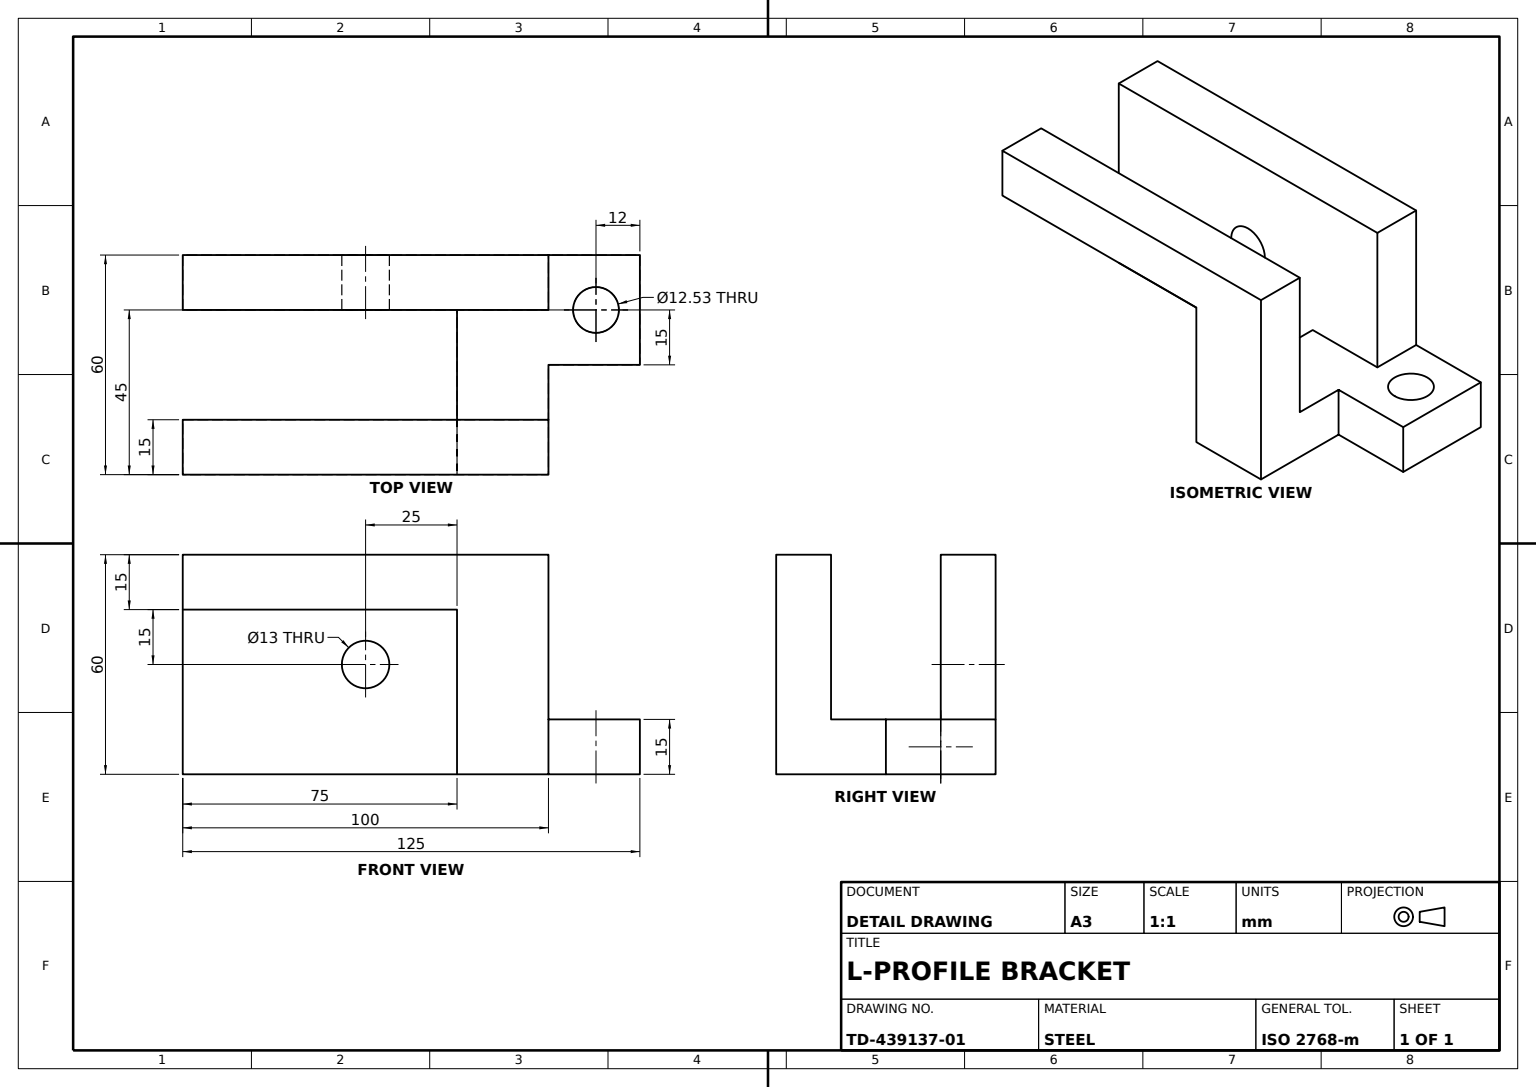
SolidWorks part; units mm, degrees
material "Plain Carbon Steel"
ref_plane "Front Plane" through (0, 0, 0) normal (0, 0, 1) x (1, 0, 0)
ref_plane "Top Plane" through (0, 0, 0) normal (0, 1, 0) x (1, 0, 0)
ref_plane "Right Plane" through (0, 0, 0) normal (1, 0, 0) x (0, 0, -1)
sketch "Channel Profile Sketch" plane through (0, 0, 0) normal (0, 0, 1) x (1, 0, 0)
  line L1 (-50, -30) -> (50, -30)
  line L2 (-50, -30) -> (-50, 30)
  line L3 (-50, 30) -> (50, 30)
  line L4 (50, -30) -> (50, 30)
  line L5 (-50, -30) -> (50, 30) construction
  line L6 (-50, 30) -> (50, -30) construction
  circle A0 centre (0, 0) radius 6.5
  point P0 (0, 0)
  dimension "D3" = 13
  dimension "D1" = 100
  dimension "D2" = 60
extrude "Channel Body" add sketch "Channel Profile Sketch" along normal blind 15
sketch "Lug Outline Sketch" plane through (0, 0, 0) normal (0, 1, 0) x (1, 0, 0)
  line L5 (50, -15) -> (50, 0) construction
  line L6 (25, -60) -> (50, -60)
  line L7 (25, -60) -> (25, 0)
  line L8 (25, 0) -> (75, 0)
  line L9 (75, -30) -> (75, 0)
  line L12 (50, 0) -> (-50, 0) construction
  line L13 (25, -60) -> (50, -60)
  line L14 (50, -60) -> (50, -30)
  line L15 (50, -30) -> (75, -30)
  circle A0 centre (63, -15) radius 6.2661
  point P0 (50, -30)
  dimension "D7" = 12.5322
  dimension "D1" = 50
  dimension "D2" = 25
  dimension "D3" = 25
  dimension "D4" = 30
  dimension "D5" = 12
  dimension "D6" = 15
  dimension "D8" = 30
sketch "Lug 1 Profile Sketch" plane through (0, -30, 0) normal (0, -1, 0) x (1, 0, 0)
  line L0 (25, 0) -> (75, 0) construction
  line L1 (75, 30) -> (75, 0) construction
  line L2 (50, 30) -> (75, 30) construction
  line L3 (50, 60) -> (50, 30) construction
  line L4 (25, 60) -> (50, 60) construction
  line L5 (25, 60) -> (25, 0) construction
  line L6 (25, 0) -> (75, 0)
  line L7 (75, 30) -> (75, 0)
  line L8 (50, 30) -> (75, 30)
  line L9 (50, 60) -> (50, 30)
  line L10 (25, 60) -> (50, 60)
  line L11 (25, 60) -> (25, 0)
  circle A0 centre (63, 15) radius 6.2661 construction
  circle A1 centre (63, 15) radius 6.2661
extrude "Pierced Lug 1" add sketch "Lug 1 Profile Sketch" against normal blind 15
sketch "Lug 2 Profile Sketch" plane through (0, 0, 60) normal (0, 0, 1) x (1, 0, 0)
  line L1 (25, -30) -> (50, -30)
  line L2 (25, -30) -> (25, 15)
  line L4 (50, -30) -> (50, 30)
  line L5 (-50, 30) -> (-50, -30) construction
  line L8 (25, 15) -> (-50, 15)
  line L9 (-50, 30) -> (-50, 15)
  line L10 (50, -30) -> (25, -30) construction
  line L11 (50, -15) -> (50, 30) construction
  line L12 (-50, 30) -> (50, 30)
  dimension "D1" = 15
  dimension "D2" = 45
extrude "Pierced Lug 2" add sketch "Lug 2 Profile Sketch" against normal blind 15
